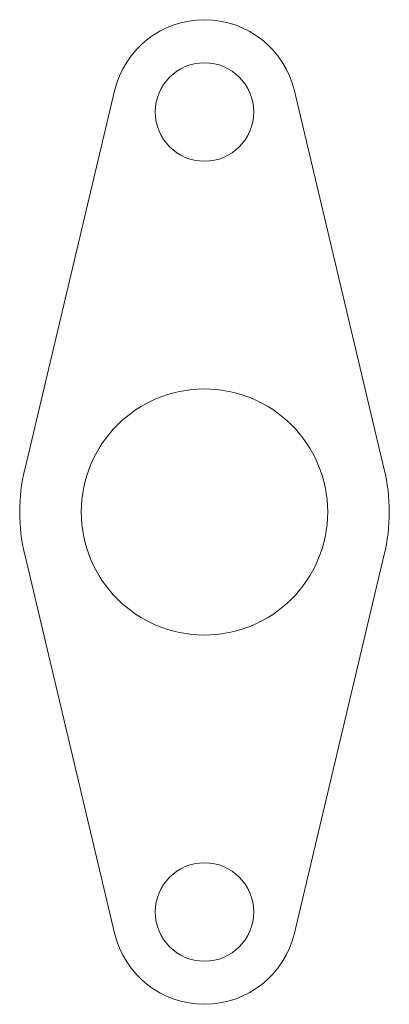
# Model space of a CAD drawing. Units: millimetres. Extents: x 3166 to 3470, y -3 to 1909.
# Tile 1 of 1: x 3165.9 to 3225.9, y 1749.1 to 1909.1. Entities that reach past the tile are written whole.
import ezdxf

# ---------------------------------------------------------------- set-up
doc = ezdxf.new("R2010")
doc.units = ezdxf.units.MM
doc.layers.add('M-CONS', color=3, linetype='Continuous', lineweight=18)

msp = doc.modelspace()

# ---------------------------------------------------------------- linework, layer by layer
at = {"layer": 'M-CONS'}
for p, q in [((3181.29, 1897.61), (3166.69, 1836.07)), ((3210.48, 1897.61), (3225.07, 1836.07)), ((3181.29, 1760.69), (3166.69, 1822.23)), ((3225.07, 1822.23), (3210.48, 1760.69))]:
    msp.add_line(p, q, dxfattribs=at)
for centre, radius in [((3195.88, 1894.15), 8), ((3195.88, 1829.15), 20), ((3195.88, 1764.15), 8)]:
    msp.add_circle(centre, radius, dxfattribs=at)
for centre, radius, start, end in [((3195.88, 1894.15), 15, 13.3424, 166.6576), ((3195.88, 1829.15), 30, 166.6576, 193.3424), ((3195.88, 1829.15), 30, 346.6576, 13.3424), ((3195.88, 1764.15), 15, 193.3424, 346.6576)]:
    msp.add_arc(centre, radius, start, end, dxfattribs=at)

doc.saveas('drawing.dxf')
